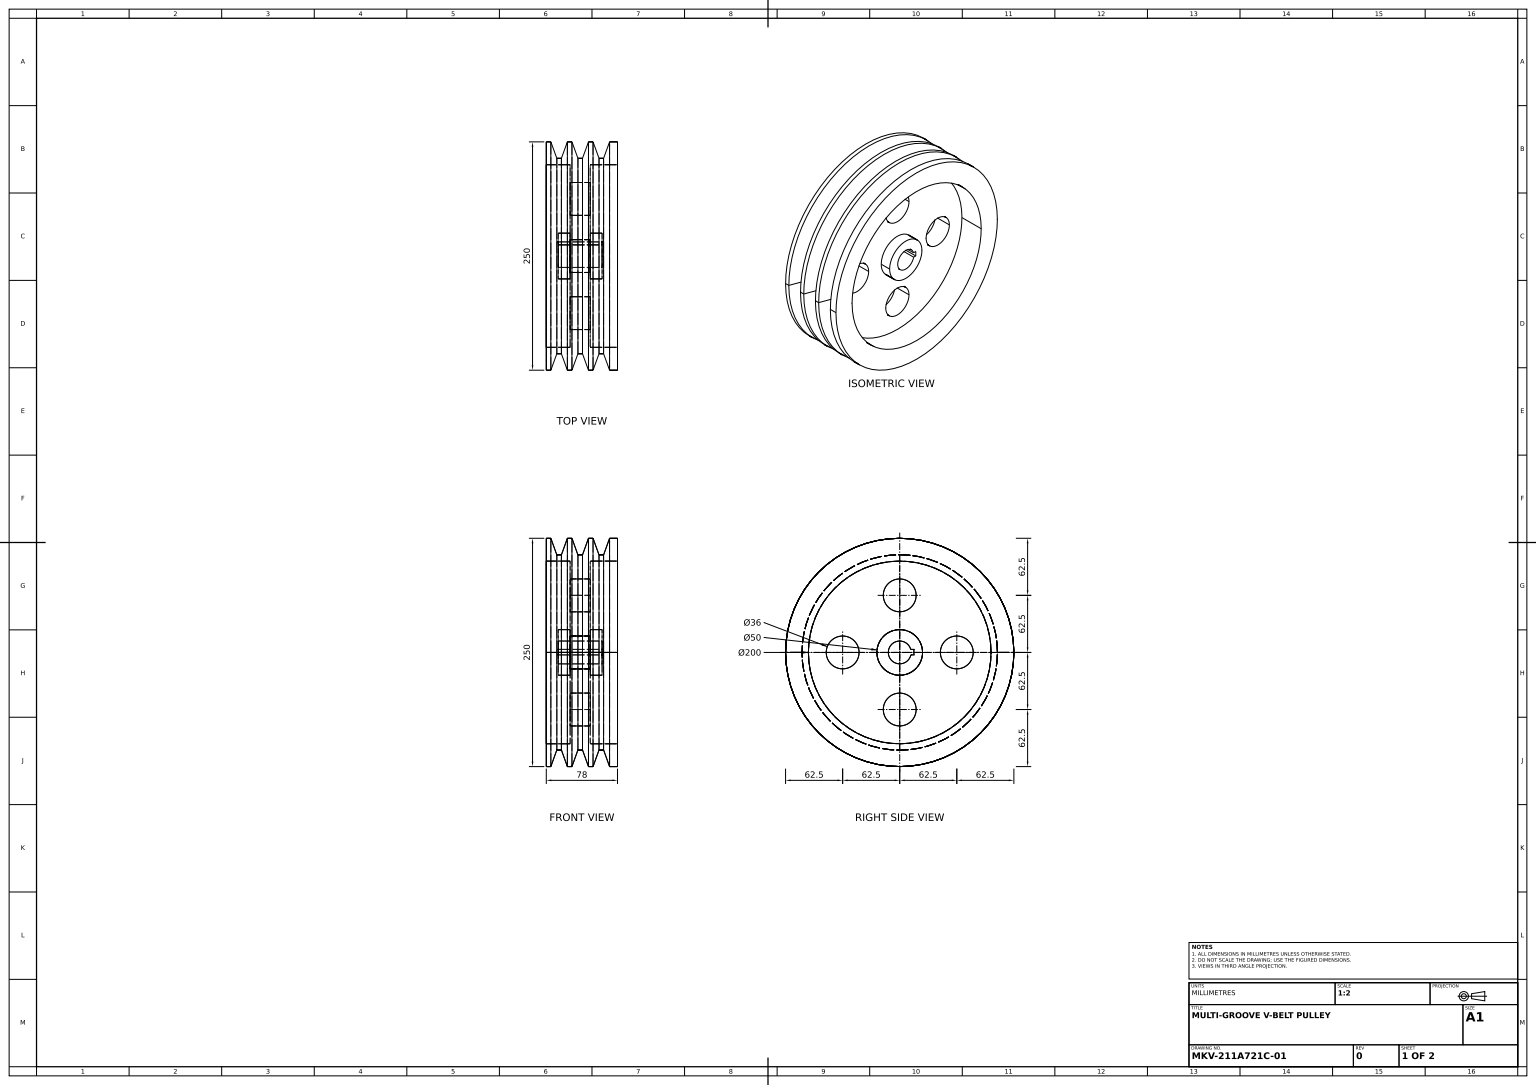
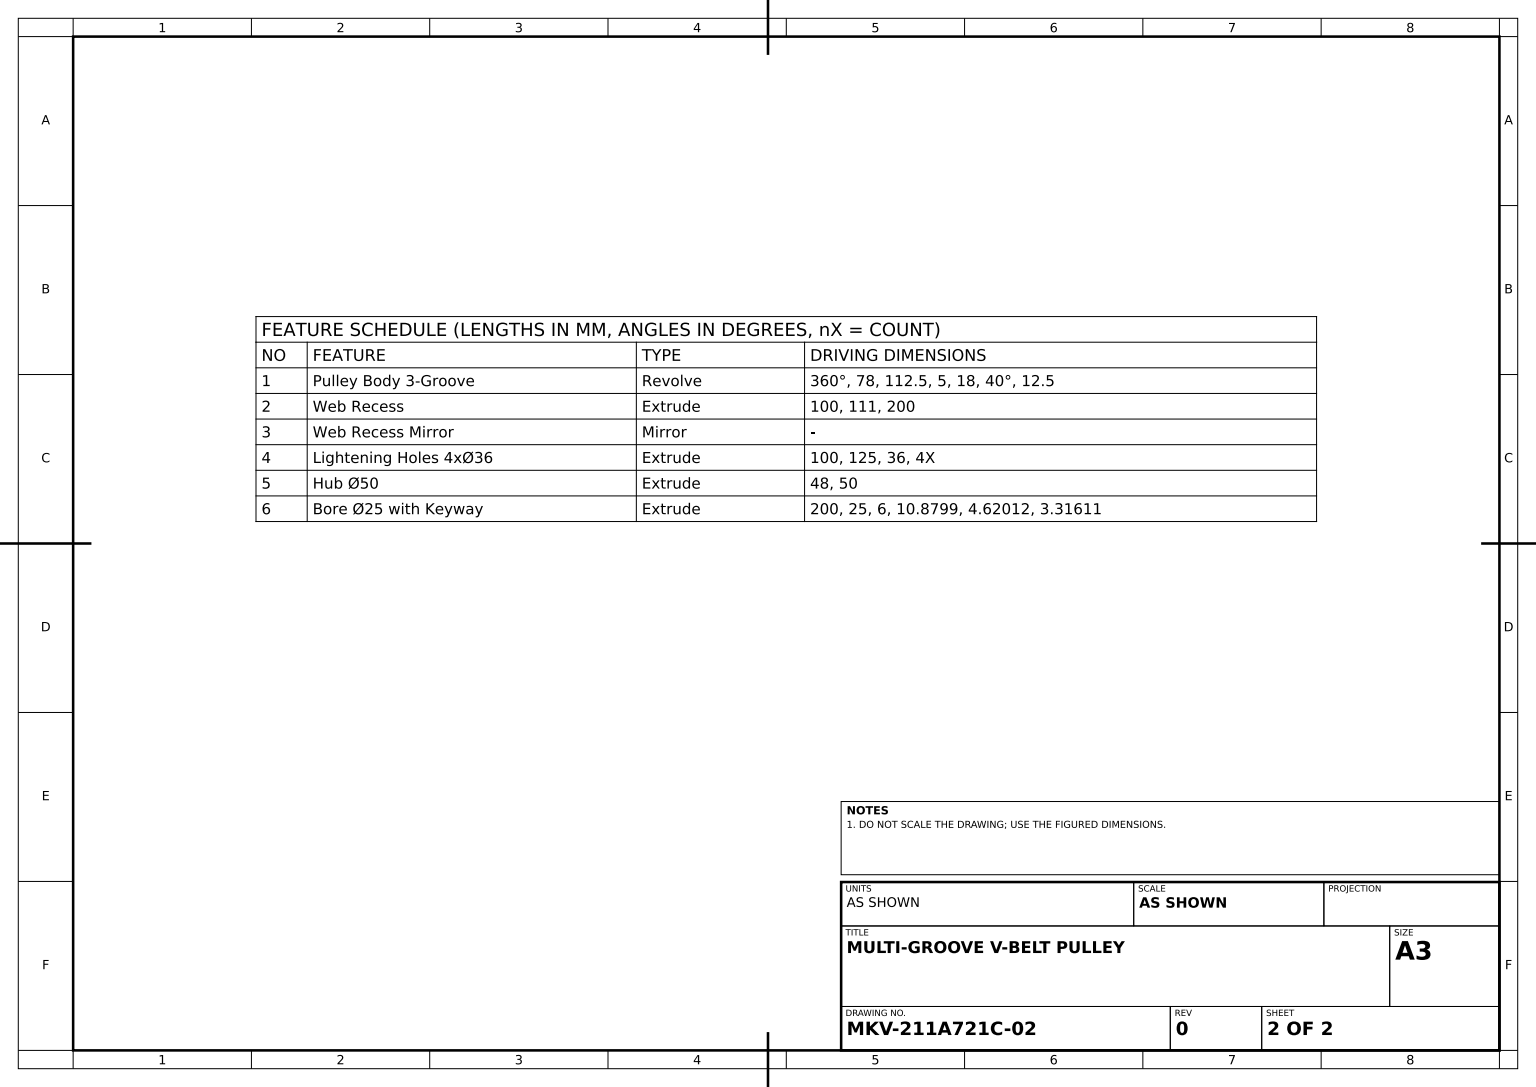
SolidWorks part; units mm, degrees
material "Plain Carbon Steel"
ref_plane "Front Plane" through (0, 0, 0) normal (0, 0, 1) x (1, 0, 0)
ref_plane "Top Plane" through (0, 0, 0) normal (0, 1, 0) x (1, 0, 0)
ref_plane "Right Plane" through (0, 0, 0) normal (1, 0, 0) x (0, 0, -1)
sketch "Pulley Profile Sketch" plane through (0, 0, 0) normal (0, 0, 1) x (1, 0, 0)
  line L0 (0, 393.9079) -> (0, -287.5297) construction
  line L1 (491.8068, 0) -> (-400.8457, 0) construction
  line L2 (-2.5, 107) -> (2.5, 107)
  line L3 (-37.1544, 125) -> (-32.1544, 125)
  line L4 (-37.1544, 125) -> (-37.1544, 12.5)
  line L5 (-37.1544, 12.5) -> (40.8456, 12.5)
  line L6 (40.8456, 125) -> (40.8456, 12.5)
  line L7 (2.5, 107) -> (9.0515, 125)
  line L8 (-2.5, 107) -> (-9.0515, 125)
  line L9 (9.0515, 125) -> (14.0515, 125)
  line L10 (-25.6029, 107) -> (-20.6029, 107)
  line L11 (-20.6029, 107) -> (-14.0515, 125)
  line L12 (-25.6029, 107) -> (-32.1544, 125)
  line L13 (-14.0515, 125) -> (-9.0515, 125)
  line L14 (20.6029, 107) -> (14.0515, 125)
  line L15 (25.6029, 107) -> (20.6029, 107)
  line L16 (25.6029, 107) -> (32.1544, 125)
  line L17 (32.1544, 125) -> (40.8456, 125)
  dimension "D1" = 78
  dimension "D2" = 112.5
  dimension "D3" = 12.5
  dimension "D4" = 5
  dimension "D5" = 18
  dimension "D6" = 40
  dimension "D7" = 5
  dimension "D8" = 5
  dimension "D9" = 5
revolve "Pulley Body 3-Groove" add sketch "Pulley Profile Sketch" angle 360 about L1
sketch "Web Recess Sketch" plane through (0, 0, 0) normal (1, 0, 0) x (0, 0, -1)
  circle A0 centre (0, 0) radius 125 construction
  circle A1 centre (0, 0) radius 125
  circle A2 centre (0, 0) radius 100
  point P0 (0, 0)
  dimension "D1" = 200
extrude "Web Recess" cut sketch "Web Recess Sketch" against normal blind 100 from offset 111 contours A2
mirror "Web Recess Mirror" about plane through (0, 0, 0) normal (1, 0, 0) of "Web Recess"
sketch "Lightening Holes Sketch" plane through (0, 0, 0) normal (1, 0, 0) x (0, 0, -1)
  circle A0 centre (0, 0) radius 62.5 construction
  circle A1 centre (62.5, 0) radius 18
  circle A2 centre (0, -62.5) radius 18
  circle A3 centre (-62.5, 0) radius 18
  circle A4 centre (0, 62.5) radius 18
  point P14 (0, 0)
  dimension "D1" = 125
  dimension "D2" = 36
  dimension "D3" = 4
extrude "Lightening Holes 4xØ36" cut sketch "Lightening Holes Sketch" against normal mid plane 100
sketch "Hub Sketch" plane through (0, 0, 0) normal (1, 0, 0) x (0, 0, -1)
  circle A0 centre (0, 0) radius 25
  dimension "D1" = 50
extrude "Hub Ø50" add sketch "Hub Sketch" along normal mid plane 48
sketch "Bore Keyway Sketch" plane through (0, 0, 0) normal (1, 0, 0) x (0, 0, -1)
  line L1 (4.6201, 3.3161) -> (15.5, 3.3161)
  line L2 (4.6201, 3.3161) -> (4.6201, -2.6839)
  line L3 (4.6201, -2.6839) -> (15.5, -2.6839)
  line L4 (15.5, 3.3161) -> (15.5, -2.6839)
  circle A0 centre (0, 0) radius 12.5
  dimension "D1" = 25
  dimension "D2" = 6
  dimension "D3" = 10.8799
  dimension "D4" = 4.6201
  dimension "D5" = 3.3161
extrude "Bore Ø25 with Keyway" cut sketch "Bore Keyway Sketch" against normal mid plane 200 contours L3 L4 L1 L2 | A0
